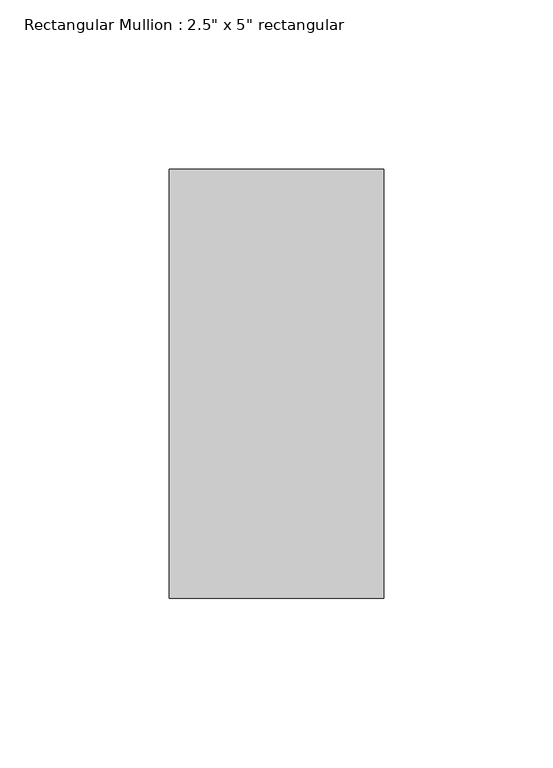
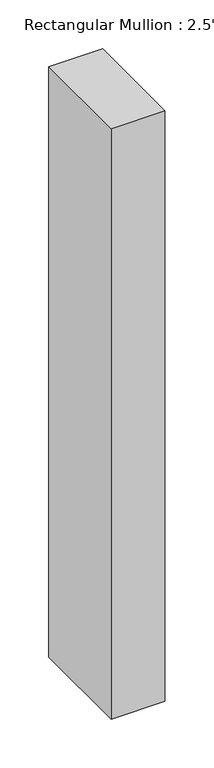
"""IFC4 building model written with IfcOpenShell, lengths in millimetres: member geometry."""

from ifc_helpers import new_model, si_unit, frame, origin, place, context, project, spatial, polyline, outline, extrude, source, transform, mapped, element, save


def member_dae533be(model_context):
    return source(origin(), model_context, "Body", "SweptSolid", [
        extrude(outline(polyline([(0.0, 63.5), (0.0, -63.5), (-63.5, -63.5), (-63.5, 63.5), (0.0, 63.5)])), frame((0.0, 0.0, -736.5781229), z_axis=(0.0, 0.0, 1.0), x_axis=(1.0, 0.0, 0.0)), (0.0, 0.0, 1.0), 736.5781229),
    ])


if __name__ == "__main__":
    model = new_model("IFC4")
    model_context = context("Model", 3, world=origin())
    ifc_project = project(units=[si_unit("LENGTHUNIT", "METRE", prefix="MILLI")], contexts=[model_context])
    site = spatial("IfcSite", under=ifc_project)
    building = spatial("IfcBuilding", under=site)
    placement = place(None, origin())
    member_shape = member_dae533be(model_context)
    element("IfcMember", 1, ObjectType="Rectangular Mullion : 2.5\" x 5\" rectangular", at=placement, inside=building, context=model_context, shape_type="MappedRepresentation", body=[
        mapped(member_shape, transform((0.0, 0.0, 0.0), x_axis=(1.0, 0.0, 0.0), y_axis=(0.0, 1.0, 0.0), z_axis=(0.0, 0.0, 1.0))),
    ])
    save(model, "model.ifc")

# Revit data of these elements
# Type "Rectangular Mullion : 2.5\" x 5\" rectangular"
#   built-in parameter 1007304 = 0.416667 (stored number, unit not read)
#   built-in parameter 1007301 = 0.104167 (stored number, unit not read)
#   built-in parameter 1007300 = 0.104167 (stored number, unit not read)
# Element 1 (IfcMember, "Rectangular Mullion : 2.5\" x 5\" rectangular")
#   Materials on its faces: "Aluminum"
# Materials
#   "Aluminum": class "Metal", colour RGB 247 247 247, transparency 0, Description = "Aluminum 6061", Cost = 0
